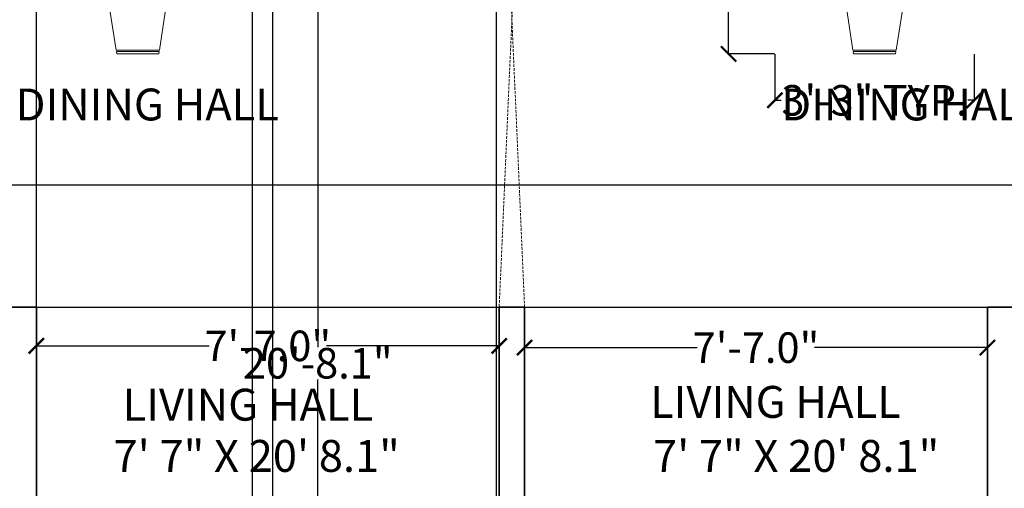
# Model space of a CAD drawing. Units: inches. Extents: x 844 to 2234, y 346 to 1084.
# Tile 42 of 93: x 1093 to 1287, y 731 to 823. Entities that reach past the tile are written whole.
import ezdxf

# ---------------------------------------------------------------- set-up
doc = ezdxf.new("R2010")
doc.units = ezdxf.units.IN
doc.header["$MEASUREMENT"] = 0
doc.linetypes.add('DASHED', pattern=[0.75, 0.5, -0.25])
for name, color, linetype, lineweight in [('A-ANNO-DIMS', 2, 'Continuous', 18), ('A-AREA-IDEN', 7, 'Continuous', 18), ('A-WALL', 7, 'Continuous', 35), ('A-WALL-OVHD', 7, 'DASHED', 18), ('furniture', 8, 'Continuous', 18)]:
    doc.layers.add(name, color=color, linetype=linetype, lineweight=lineweight)
doc.styles.add('ATTR', font='romans.shx', dxfattribs={"width": 0.8, "height": 0.7})
doc.styles.get("Standard").update_dxf_attribs({"font": 'arial.ttf'})
doc.dimstyles.get("Standard").update_dxf_attribs({"dimtxt": 6, "dimasz": 3, "dimexe": 0.18, "dimexo": 0.0625, "dimgap": 0.09, "dimtad": 0, "dimtih": 1, "dimtoh": 1, "dimdec": 1, "dimzin": 0, "dimdsep": 46, "dimlunit": 3, "dimtxsty": 'Standard', "dimblk": 'ARCHTICK', "dimcen": 0.09, "dimadec": 0, "dimazin": 0, "dimtfac": 1, "dimtdec": 1, "dimtofl": 0, "dimtmove": 0, "dimatfit": 3, "dimfxl": 1, "dimtolj": 1, "dimtzin": 0, "dimarcsym": 0})

# ---------------------------------------------------------------- blocks, each defined once
blk = doc.blocks.new('DIN42X84')
for p, q in [((-34.5377, 37.999999), (-34.6939, 37.000439)), ((-34.5377, 37.999999), (-18.5377, 37.999999)), ((-18.3814, 36.999659), (-18.5377, 37.999999)), ((-8.0001, 37.999999), (-8.1562, 37.000439)), ((-8.0001, 37.999999), (7.9999, 37.999999)), ((8.1562, 36.999659), (7.9999, 37.999999)), ((18.3813, 36.999659), (18.5376, 37.999999)), ((34.5376, 37.999999), (18.5376, 37.999999)), ((34.5376, 37.999999), (34.6938, 37.000439)), ((-34.772, 36.500609), (-37.0377, 21.999999)), ((-34.7681, 36.499999), (-18.2986, 36.499999)), ((-18.3793, 36.999999), (-34.6911, 36.999999)), ((-16.0377, 21.999999), (-18.3032, 36.499269)), ((-8.2343, 36.500609), (-10.5001, 21.999999)), ((-8.2305, 36.499999), (8.2391, 36.499999)), ((8.1584, 36.999999), (-8.1535, 36.999999)), ((10.4999, 21.999999), (8.2344, 36.499269)), ((16.0376, 21.999999), (18.3031, 36.499269)), ((34.768, 36.499999), (18.2985, 36.499999)), ((18.3792, 36.999999), (34.691, 36.999999)), ((34.7719, 36.500609), (37.0376, 21.999999)), ((-57.9997, 8.156299), (-59, 7.999989)), ((-59, -8.000011), (-59, 7.999989)), ((-58, 8.158429), (-58, -8.153391)), ((-57.5, -8.230411), (-57.5, 8.239139)), ((-43, 10.499989), (-57.4993, 8.234489)), ((43, 10.499989), (57.4992, 8.234489)), ((57.5, -8.230411), (57.5, 8.239139)), ((57.9996, 8.156299), (59, 7.999989)), ((58, 8.158429), (58, -8.153391)), ((59, -8.000011), (59, 7.999989)), ((-59, -8.000011), (-58.0005, -8.156181)), ((-57.5007, -8.234271), (-43, -10.500011)), ((57.5006, -8.234271), (43, -10.500011)), ((59, -8.000011), (58.0004, -8.156181)), ((-42, -21.000001), (42, -21.000001)), ((-34.772, -36.50061), (-37.0377, -22.000001)), ((-16.0377, -22.000001), (-18.3032, -36.499267)), ((-8.2343, -36.50061), (-10.5001, -22.000001)), ((10.4999, -22.000001), (8.2344, -36.499267)), ((16.0376, -22.000001), (18.3031, -36.499267)), ((34.7719, -36.50061), (37.0376, -22.000001)), ((-34.7681, -36.499999), (-18.2986, -36.499999)), ((-34.5377, -37.999999), (-34.6939, -37.000442)), ((-18.3793, -36.999999), (-34.6911, -36.999999)), ((-18.3814, -36.999664), (-18.5377, -37.999999)), ((-8.2305, -36.499999), (8.2391, -36.499999)), ((-8.0001, -37.999999), (-8.1562, -37.000442)), ((8.1584, -36.999999), (-8.1535, -36.999999)), ((8.1562, -36.999664), (7.9999, -37.999999)), ((34.768, -36.499999), (18.2985, -36.499999)), ((18.3792, -36.999999), (34.691, -36.999999)), ((18.3813, -36.999664), (18.5376, -37.999999)), ((34.5376, -37.999999), (34.6938, -37.000442)), ((-34.5377, -37.999999), (-18.5377, -37.999999)), ((-8.0001, -37.999999), (7.9999, -37.999999)), ((34.5376, -37.999999), (18.5376, -37.999999))]:
    blk.add_line(p, q)
for points in [[(-42, -21.000001), (-42, 20.999989), (42, 20.999989), (42, -21.000001)], [(-42, 16.999989), (-40.5974, 16.672209), (-39.2569, 16.395939), (-37.9668, 16.166109), (-36.7153, 15.977689), (-35.4906, 15.825599), (-34.281, 15.704799), (-33.0745, 15.610229), (-31.8595, 15.536839), (-30.6267, 15.480229), (-29.3778, 15.438619), (-28.117, 15.410889), (-26.8486, 15.395929), (-25.5767, 15.392599), (-24.3058, 15.399809), (-23.0399, 15.416409), (-21.7833, 15.441309), (-20.5384, 15.473619), (-19.2994, 15.513549), (-18.0587, 15.561549), (-16.8087, 15.618049), (-15.5417, 15.683499), (-14.25, 15.758369), (-12.9261, 15.843079), (-11.5622, 15.938089), (-10.1541, 16.043559), (-8.7108, 16.158419), (-7.2445, 16.281349), (-5.7675, 16.410999), (-4.2923, 16.546019), (-2.8311, 16.685069), (-1.3963, 16.826809), (0, 16.969889), (1.3474, 17.113339), (2.6447, 17.257689), (3.8928, 17.403829), (5.0924, 17.552659), (6.2444, 17.705069), (7.3498, 17.861959), (8.4092, 18.024219), (9.4237, 18.192759), (10.3952, 18.367629), (11.3311, 18.545639), (12.2397, 18.722759), (13.1297, 18.894949), (14.0095, 19.058179), (14.8876, 19.208429), (15.7725, 19.341659), (16.6727, 19.453839), (17.5977, 19.541909), (18.5617, 19.606689), (19.5795, 19.649979), (20.6664, 19.673569), (21.8374, 19.679239), (23.1076, 19.668789), (24.492, 19.644009), (26.0058, 19.606689), (27.6589, 19.554579), (29.4413, 19.469229), (31.3377, 19.328169), (33.3331, 19.108889), (35.4121, 18.788919), (37.5598, 18.345779), (39.7608, 17.756959), (42, 16.999989)], [(42, 12.999999), (39.3635, 13.704689), (36.9303, 14.232849), (34.6868, 14.608169), (32.6195, 14.854319), (30.7149, 14.994989), (28.9596, 15.053859), (27.34, 15.054629), (25.8427, 15.020959), (24.4543, 14.972439), (23.1628, 14.912279), (21.9562, 14.839589), (20.8227, 14.753449), (19.7504, 14.652989), (18.7273, 14.537299), (17.7416, 14.405489), (16.7814, 14.256669), (15.8348, 14.090369), (14.8899, 13.907959), (13.9348, 13.711209), (12.9575, 13.501929), (11.9464, 13.281899), (10.8893, 13.052909), (9.7745, 12.816759), (8.59, 12.575229), (7.3261, 12.330049), (5.9815, 12.082619), (4.557, 11.834299), (3.0536, 11.586429), (1.472, 11.340349), (-0.187, 11.097409), (-1.9223, 10.858939), (-3.7333, 10.626289), (-5.6141, 10.400739), (-7.539, 10.183249), (-9.4776, 9.974709), (-11.3991, 9.776019), (-13.2731, 9.588079), (-15.0689, 9.411789), (-16.756, 9.248039), (-18.3038, 9.097709), (-19.6928, 8.961719), (-20.9483, 8.840959), (-22.1065, 8.736319), (-23.2037, 8.648689), (-24.2763, 8.578979), (-25.3606, 8.528079), (-26.4928, 8.496879), (-27.7094, 8.486279), (-29.0411, 8.496689), (-30.4965, 8.526549), (-32.0787, 8.573829), (-33.7908, 8.636479), (-35.6359, 8.712459), (-37.6171, 8.799739), (-39.7374, 8.896259), (-42, 8.999999)], [(-42, 0.999999), (-39.2567, 1.059739), (-36.6668, 1.127399), (-34.2177, 1.203389), (-31.897, 1.288099), (-29.6923, 1.381949), (-27.5912, 1.485329), (-25.5812, 1.598659), (-23.65, 1.722319), (-21.7874, 1.856519), (-19.9935, 2.000569), (-18.2704, 2.153579), (-16.6207, 2.314649), (-15.0465, 2.482879), (-13.5503, 2.657379), (-12.1344, 2.837259), (-10.8011, 3.021619), (-9.5514, 3.209479), (-8.3812, 3.399579), (-7.2848, 3.590579), (-6.2569, 3.781129), (-5.2918, 3.969889), (-4.384, 4.155509), (-3.5281, 4.336659), (-2.7184, 4.511979), (-1.9505, 4.680359), (-1.2233, 4.841579), (-0.5369, 4.995629), (0.1087, 5.142519), (0.7135, 5.282239), (1.2776, 5.414799), (1.8009, 5.540189), (2.2834, 5.658409), (2.7259, 5.769699), (3.1323, 5.875159), (3.5073, 5.976139), (3.8555, 6.073989), (4.1816, 6.170049), (4.4904, 6.265659), (4.7863, 6.362169), (5.0742, 6.460919), (5.3584, 6.563099), (5.6417, 6.669299), (5.9267, 6.779989), (6.216, 6.895609), (6.512, 7.016589), (6.8174, 7.143399), (7.1347, 7.276479), (7.4664, 7.416279), (7.8159, 7.563169), (8.1896, 7.717219), (8.5948, 7.878439), (9.0386, 8.046819), (9.5282, 8.222369), (10.071, 8.405079), (10.674, 8.594959), (11.3446, 8.791999), (12.0866, 8.995459), (12.8902, 9.201609), (13.7421, 9.405969), (14.6294, 9.604059), (15.5387, 9.791399), (16.4569, 9.963509), (17.3709, 10.115919), (18.2674, 10.244149), (19.1361, 10.344989), (19.9772, 10.420299), (20.7936, 10.473209), (21.5884, 10.506879), (22.3645, 10.524419), (23.1248, 10.528969), (23.8725, 10.523669), (24.6103, 10.511649), (25.3403, 10.495379), (26.0601, 10.474629), (26.7663, 10.448509), (27.4556, 10.416119), (28.1244, 10.376559), (28.7695, 10.328939), (29.3873, 10.272359), (29.9746, 10.205939), (30.5293, 10.129059), (31.0552, 10.042329), (31.5572, 9.946639), (32.0406, 9.842899), (32.5104, 9.731989), (32.9716, 9.614799), (33.4295, 9.492249), (33.8891, 9.365219), (34.3546, 9.234229), (34.8266, 9.098309), (35.3051, 8.956129), (35.7897, 8.806329), (36.2802, 8.647569), (36.7765, 8.478519), (37.2783, 8.297819), (37.7854, 8.104139), (38.2976, 7.894309), (38.8146, 7.657969), (39.3361, 7.382899), (39.8617, 7.056919), (40.3912, 6.667829), (40.9243, 6.203449), (41.4607, 5.651569), (42, 4.999999)], [(42, 0.999999), (35.1214, 2.295539), (25.1178, 2.983399), (7.9376, 2.295539), (0.3261, 1.149099), (-6.6329, -0.226611), (-18.3763, -2.978061), (-22.0733, -3.895201), (-27.5101, -4.583071), (-32.9468, -4.583071), (-35.339, -4.583071), (-38.3836, -4.353771), (-40.3408, -3.665921), (-42, -3.000001)], [(42, -3.000001), (38.9344, -2.781351), (35.8829, -2.650251), (32.8567, -2.595491), (29.8672, -2.605821), (26.9257, -2.670031), (24.0436, -2.776881), (21.2323, -2.915141), (18.5031, -3.073591), (15.8668, -3.242611), (13.3327, -3.419021), (10.9095, -3.601241), (8.6059, -3.787731), (6.4305, -3.976901), (4.3921, -4.167191), (2.4994, -4.357031), (0.7611, -4.544851), (-0.8196, -4.729651), (-2.2614, -4.912671), (-3.5885, -5.095681), (-4.8252, -5.280481), (-5.9956, -5.468861), (-7.1239, -5.662621), (-8.2344, -5.863551), (-9.3513, -6.073431), (-10.4925, -6.293091), (-11.6511, -6.519461), (-12.814, -6.748531), (-13.968, -6.976251), (-15.0999, -7.198591), (-16.1965, -7.411531), (-17.2447, -7.611041), (-18.2313, -7.793081), (-19.1472, -7.954521), (-19.9994, -8.095811), (-20.7989, -8.218291), (-21.5568, -8.323311), (-22.2841, -8.412201), (-22.9919, -8.486311), (-23.6912, -8.546991), (-24.393, -8.595581), (-25.1087, -8.632751), (-25.8513, -8.656491), (-26.6337, -8.664101), (-27.4693, -8.652901), (-28.3711, -8.620211), (-29.3523, -8.563341), (-30.4262, -8.479601), (-31.6057, -8.366301), (-32.8956, -8.222561), (-34.2657, -8.054761), (-35.6772, -7.871051), (-37.0913, -7.679611), (-38.4695, -7.488621), (-39.7728, -7.306241), (-40.9626, -7.140641), (-42, -7.000001)], [(-42, -15.000001), (-38.4722, -15.350691), (-35.3039, -15.623741), (-32.4544, -15.828971), (-29.8831, -15.976191), (-27.5493, -16.075201), (-25.4123, -16.135831), (-23.4313, -16.167881), (-21.5659, -16.181151), (-19.7812, -16.183881), (-18.0665, -16.177871), (-16.4173, -16.163351), (-14.8288, -16.140551), (-13.2964, -16.109691), (-11.8154, -16.070991), (-10.3811, -16.024671), (-8.9888, -15.970971), (-7.6345, -15.909991), (-6.3163, -15.841401), (-5.0329, -15.764751), (-3.7831, -15.679591), (-2.5656, -15.585471), (-1.3791, -15.481951), (-0.2223, -15.368571), (0.9061, -15.244901), (2.0079, -15.110631), (3.0876, -14.966051), (4.1503, -14.811631), (5.2011, -14.647801), (6.2451, -14.475011), (7.2875, -14.293721), (8.3332, -14.104361), (9.3874, -13.907391), (10.4544, -13.703711), (11.5349, -13.495991), (12.6291, -13.287381), (13.7368, -13.081011), (14.8581, -12.880011), (15.9931, -12.687521), (17.1416, -12.506671), (18.3037, -12.340601), (19.4778, -12.191771), (20.6562, -12.059961), (21.8295, -11.944271), (22.9884, -11.843811), (24.1234, -11.757681), (25.2254, -11.684981), (26.2848, -11.624831), (27.2925, -11.576311), (28.2412, -11.538551), (29.1325, -11.510631), (29.9703, -11.491671), (30.7584, -11.480781), (31.5007, -11.477041), (32.2009, -11.479581), (32.8628, -11.487491), (33.4904, -11.499881), (34.0874, -11.515741), (34.6576, -11.533621), (35.2049, -11.551941), (35.733, -11.569151), (36.2459, -11.583661), (36.7473, -11.593931), (37.2411, -11.598371), (37.7311, -11.595421), (38.2211, -11.583281), (38.7152, -11.559251), (39.2177, -11.520361), (39.7326, -11.463671), (40.2641, -11.386241), (40.8164, -11.285111), (41.3937, -11.157351), (42, -11.000001)]]:
    blk.add_lwpolyline(points)
for centre, start, end in [((-36.0377, 21.999999), 180, 270), ((-17.0377, 21.999999), 270, 0), ((-9.5001, 21.999999), 180, 270), ((9.4999, 21.999999), 270, 0), ((17.0376, 21.999999), 180, 270), ((36.0376, 21.999999), 270, 0), ((-43, 9.499989), 0.00000068, 90), ((43, 9.499989), 90, 180), ((-43, -9.500011), 270, 0.00000068), ((43, -9.500011), 180, 270), ((-36.0377, -22.000001), 90, 180), ((-17.0377, -22.000001), 0, 90), ((-9.5001, -22.000001), 90, 180), ((9.4999, -22.000001), 0, 90), ((17.0376, -22.000001), 90, 180), ((36.0376, -22.000001), 0, 90)]:
    blk.add_arc(centre, 1, start, end)
at = {"style": 'ATTR', "width": 0.8, "flags": 9}
blk.add_attdef('ESTCODE', (0, 0), '', height=0.7, dxfattribs=at)
blk = doc.blocks.new('_ArchTick')
at = {"color": 0, "linetype": 'ByBlock', "const_width": 0.15}
blk.add_lwpolyline([(-0.5, -0.5), (0.5, 0.5)], dxfattribs=at)
blk = doc.blocks.new('*D49')
at = {"layer": 'A-ANNO-DIMS', "color": 0, "lineweight": -2, "transparency": 16777216}
for p, q in [((1192.62, 758.39), (1192.62, 758.51)), ((1192.62, 758.33), (1226.58, 758.33)), ((1283.62, 758.33), (1249.65, 758.33)), ((1283.62, 758.39), (1283.62, 758.51))]:
    blk.add_line(p, q, dxfattribs=at)
at = {"layer": 'Defpoints', "color": 0, "transparency": 16777216}
for p in [(1192.62, 758.33), (1192.62, 758.33), (1283.62, 758.33)]:
    blk.add_point(p, dxfattribs=at)
at = {"layer": 'A-ANNO-DIMS', "color": 0, "lineweight": -2, "transparency": 16777216, "xscale": 3, "yscale": 3, "zscale": 3, "rotation": 180}
blk.add_blockref('_ArchTick', (1192.62, 758.33), dxfattribs=at)
at = {"layer": 'A-ANNO-DIMS', "color": 0, "lineweight": -2, "transparency": 16777216, "xscale": 3, "yscale": 3, "zscale": 3}
blk.add_blockref('_ArchTick', (1283.62, 758.33), dxfattribs=at)
at = {"layer": 'A-ANNO-DIMS', "color": 0, "transparency": 16777216, "insert": (1238.12, 758.33), "char_height": 6, "attachment_point": 5}
blk.add_mtext('\\A1;7\'-7.0"', dxfattribs=at)
blk = doc.blocks.new('*D53')
at = {"layer": 'A-ANNO-DIMS', "color": 0, "lineweight": -2, "transparency": 16777216}
for p, q in [((1096.62, 758.67), (1130.58, 758.67)), ((1096.62, 758.6), (1096.62, 758.49)), ((1187.62, 758.67), (1153.65, 758.67)), ((1187.62, 758.73), (1187.62, 758.85))]:
    blk.add_line(p, q, dxfattribs=at)
at = {"layer": 'Defpoints', "color": 0, "transparency": 16777216}
for p in [(1096.62, 758.67), (1187.62, 758.67), (1187.62, 758.67)]:
    blk.add_point(p, dxfattribs=at)
at = {"layer": 'A-ANNO-DIMS', "color": 0, "lineweight": -2, "transparency": 16777216, "xscale": 3, "yscale": 3, "zscale": 3, "rotation": 180}
blk.add_blockref('_ArchTick', (1096.62, 758.67), dxfattribs=at)
at = {"layer": 'A-ANNO-DIMS', "color": 0, "lineweight": -2, "transparency": 16777216, "xscale": 3, "yscale": 3, "zscale": 3}
blk.add_blockref('_ArchTick', (1187.62, 758.67), dxfattribs=at)
at = {"layer": 'A-ANNO-DIMS', "color": 0, "transparency": 16777216, "insert": (1142.12, 758.67), "char_height": 6, "attachment_point": 5}
blk.add_mtext('\\A1;7\'-7.0"', dxfattribs=at)
blk = doc.blocks.new('*D54')
at = {"layer": 'A-ANNO-DIMS', "color": 0, "lineweight": -2, "transparency": 16777216}
for p, q in [((1139.68, 879.31), (1152.12, 879.31)), ((1151.94, 879.31), (1151.94, 758.4)), ((1151.94, 631.18), (1151.94, 752.09)), ((1139.68, 631.18), (1152.12, 631.18))]:
    blk.add_line(p, q, dxfattribs=at)
at = {"layer": 'Defpoints', "color": 0, "transparency": 16777216}
for p in [(1139.62, 879.31), (1139.62, 631.18), (1151.94, 631.18)]:
    blk.add_point(p, dxfattribs=at)
at = {"layer": 'A-ANNO-DIMS', "color": 0, "lineweight": -2, "transparency": 16777216, "xscale": 3, "yscale": 3, "zscale": 3}
for p, rotation in [((1151.94, 879.31), 90), ((1151.94, 631.18), 270)]:
    blk.add_blockref('_ArchTick', p, dxfattribs=dict(at, rotation=rotation))
at = {"layer": 'A-ANNO-DIMS', "color": 0, "transparency": 16777216, "insert": (1151.94, 755.25), "char_height": 6, "attachment_point": 5}
blk.add_mtext('\\A1;20\'-8.1"', dxfattribs=at)
blk = doc.blocks.new('*D119')
at = {"layer": 'A-ANNO-DIMS', "color": 0, "lineweight": -2, "transparency": 16777216}
for p, q in [((1241.78, 876.89), (1232.54, 876.89)), ((1232.72, 876.89), (1232.72, 849.68)), ((1232.72, 816.08), (1232.72, 843.29)), ((1241.78, 816.08), (1232.54, 816.08))]:
    blk.add_line(p, q, dxfattribs=at)
at = {"layer": 'Defpoints', "color": 0, "transparency": 16777216}
for p in [(1232.72, 876.89), (1241.84, 876.89), (1241.84, 816.08)]:
    blk.add_point(p, dxfattribs=at)
at = {"layer": 'A-ANNO-DIMS', "color": 0, "lineweight": -2, "transparency": 16777216, "xscale": 3, "yscale": 3, "zscale": 3}
for p, rotation in [((1232.72, 876.89), 90), ((1232.72, 816.08), 270)]:
    blk.add_blockref('_ArchTick', p, dxfattribs=dict(at, rotation=rotation))
at = {"layer": 'A-ANNO-DIMS', "color": 0, "transparency": 16777216, "insert": (1232.72, 846.48), "char_height": 6, "attachment_point": 5}
blk.add_mtext('\\A1;DINING SET 5\'-1" TYP.', dxfattribs=at)
blk = doc.blocks.new('*D120')
at = {"layer": 'A-ANNO-DIMS', "color": 0, "lineweight": -2, "transparency": 16777216}
for p, q in [((1241.84, 816.01), (1241.84, 806.78)), ((1281.01, 816.01), (1281.01, 806.78)), ((1241.84, 806.96), (1243.05, 806.96)), ((1281.01, 806.96), (1279.8, 806.96))]:
    blk.add_line(p, q, dxfattribs=at)
at = {"layer": 'Defpoints', "color": 0, "transparency": 16777216}
for p in [(1241.84, 816.08), (1281.01, 816.08), (1241.84, 806.96)]:
    blk.add_point(p, dxfattribs=at)
at = {"layer": 'A-ANNO-DIMS', "color": 0, "lineweight": -2, "transparency": 16777216, "xscale": 3, "yscale": 3, "zscale": 3, "rotation": 180}
blk.add_blockref('_ArchTick', (1241.84, 806.96), dxfattribs=at)
at = {"layer": 'A-ANNO-DIMS', "color": 0, "lineweight": -2, "transparency": 16777216, "xscale": 3, "yscale": 3, "zscale": 3}
blk.add_blockref('_ArchTick', (1281.01, 806.96), dxfattribs=at)
at = {"layer": 'A-ANNO-DIMS', "color": 0, "transparency": 16777216, "insert": (1261.43, 806.96), "char_height": 6, "attachment_point": 5}
blk.add_mtext('\\A1;3\'-3" TYP.', dxfattribs=at)
blk = doc.blocks.new('*D143')
at = {"layer": 'A-ANNO-DIMS', "color": 0, "lineweight": -2, "transparency": 16777216}
for p, q in [((1139.12, 430.37), (1139.12, 1074.74)), ((1139.12, 1074.56), (1154.93, 1074.56)), ((1187.12, 1074.56), (1171.3, 1074.56)), ((1187.12, 430.37), (1187.12, 1074.74))]:
    blk.add_line(p, q, dxfattribs=at)
at = {"layer": 'Defpoints', "color": 0, "transparency": 16777216}
for p in [(1187.12, 1074.56), (1139.12, 430.31), (1187.12, 430.31)]:
    blk.add_point(p, dxfattribs=at)
at = {"layer": 'A-ANNO-DIMS', "color": 0, "lineweight": -2, "transparency": 16777216, "xscale": 3, "yscale": 3, "zscale": 3, "rotation": 180}
blk.add_blockref('_ArchTick', (1139.12, 1074.56), dxfattribs=at)
at = {"layer": 'A-ANNO-DIMS', "color": 0, "lineweight": -2, "transparency": 16777216, "xscale": 3, "yscale": 3, "zscale": 3}
blk.add_blockref('_ArchTick', (1187.12, 1074.56), dxfattribs=at)
at = {"layer": 'A-ANNO-DIMS', "color": 0, "transparency": 16777216, "insert": (1163.12, 1074.56), "char_height": 6, "attachment_point": 5}
blk.add_mtext('\\A1;4\'-0"', dxfattribs=at)
blk = doc.blocks.new('*D144')
at = {"layer": 'A-ANNO-DIMS', "color": 0, "lineweight": -2, "transparency": 16777216}
for p, q in [((1096.62, 439.37), (1096.62, 1074.74)), ((1096.62, 1074.56), (1102.48, 1074.56)), ((1143.12, 1074.56), (1137.25, 1074.56)), ((1143.12, 492.37), (1143.12, 1074.74))]:
    blk.add_line(p, q, dxfattribs=at)
at = {"layer": 'Defpoints', "color": 0, "transparency": 16777216}
for p in [(1143.12, 1074.56), (1143.12, 492.31), (1096.62, 439.31)]:
    blk.add_point(p, dxfattribs=at)
at = {"layer": 'A-ANNO-DIMS', "color": 0, "lineweight": -2, "transparency": 16777216, "xscale": 3, "yscale": 3, "zscale": 3, "rotation": 180}
blk.add_blockref('_ArchTick', (1096.62, 1074.56), dxfattribs=at)
at = {"layer": 'A-ANNO-DIMS', "color": 0, "lineweight": -2, "transparency": 16777216, "xscale": 3, "yscale": 3, "zscale": 3}
blk.add_blockref('_ArchTick', (1143.12, 1074.56), dxfattribs=at)
at = {"layer": 'A-ANNO-DIMS', "color": 0, "transparency": 16777216, "insert": (1119.87, 1074.56), "char_height": 6, "attachment_point": 5}
blk.add_mtext('\\A1;3\'-10 1/2"', dxfattribs=at)
blk = doc.blocks.new('*D149')
at = {"layer": 'A-ANNO-DIMS', "color": 0, "lineweight": -2, "transparency": 16777216}
for p, q in [((1043.68, 790.31), (1479.05, 790.31)), ((1478.87, 790.31), (1478.87, 781.46)), ((1478.87, 766.31), (1478.87, 775.16)), ((1043.68, 766.31), (1479.05, 766.31))]:
    blk.add_line(p, q, dxfattribs=at)
at = {"layer": 'Defpoints', "color": 0, "transparency": 16777216}
for p in [(1043.62, 790.31), (1478.87, 790.31), (1043.62, 766.31)]:
    blk.add_point(p, dxfattribs=at)
at = {"layer": 'A-ANNO-DIMS', "color": 0, "lineweight": -2, "transparency": 16777216, "xscale": 3, "yscale": 3, "zscale": 3}
for p, rotation in [((1478.87, 790.31), 90), ((1478.87, 766.31), 270)]:
    blk.add_blockref('_ArchTick', p, dxfattribs=dict(at, rotation=rotation))
at = {"layer": 'A-ANNO-DIMS', "color": 0, "transparency": 16777216, "insert": (1478.87, 778.31), "char_height": 6, "attachment_point": 5}
blk.add_mtext('\\A1;2\'-0"', dxfattribs=at)

msp = doc.modelspace()

# ---------------------------------------------------------------- linework, layer by layer
at = {"layer": 'A-WALL'}
for p, q in [((1091.62, 766.31), (1096.62, 766.31)), ((1096.62, 761.31), (1096.62, 766.31)), ((1187.62, 766.31), (1192.62, 766.31)), ((1187.62, 766.31), (1187.62, 629.31)), ((1192.62, 766.31), (1192.62, 629.31)), ((1283.62, 761.31), (1283.62, 766.31)), ((1288.62, 766.31), (1283.62, 766.31)), ((1096.62, 761.31), (1096.62, 624.31)), ((1283.62, 761.31), (1283.62, 624.31))]:
    msp.add_line(p, q, dxfattribs=at)
at = {"layer": 'A-WALL-OVHD'}
for p, q in [((1192.62, 766.31), (1187.62, 879.31)), ((1192.62, 879.31), (1187.62, 766.31))]:
    msp.add_line(p, q, dxfattribs=at)

# ---------------------------------------------------------------- block references
at = {"layer": 'furniture', "xscale": 0.5153672157522483, "yscale": 0.5153672157522483, "zscale": 0.5153672157522483, "rotation": 90}
for p in [(1116.56, 846.48), (1261.43, 846.48)]:
    msp.add_blockref('DIN42X84', p, dxfattribs=at)

# ---------------------------------------------------------------- texts
at = {"layer": 'A-AREA-IDEN'}
for s, p in [('DINING HALL', (1092.53, 803)), ('DINING HALL', (1243.09, 803)), ('LIVING HALL', (1113.58, 743.97)), ('  LIVING HALL', (1213.47, 744.52)), (' 7\' 7" X 20\' 8.1"', (1109.88, 733.9)), (' 7\' 7" X 20\' 8.1"', (1215.96, 733.9))]:
    msp.add_text(s, height=6.2688, dxfattribs=at).set_placement(p)

# ---------------------------------------------------------------- dimensions: what is measured, and where the dimension line sits
at = {"layer": 'A-ANNO-DIMS'}
for base, p1, p2, override, picture, middle in [((1143.12, 1074.56), (1096.62, 439.31), (1143.12, 492.31), {"dimdec": 1, "dimlfac": 1, "dimrnd": 0, "dimzin": 1, "dimdsep": 46, "dimlunit": 4, "dimfrac": 2}, '*D144', (1119.87, 1074.56)), ((1187.12, 1074.56), (1139.12, 430.31), (1187.12, 430.31), {"dimdec": 1, "dimlfac": 1, "dimrnd": 0, "dimzin": 1, "dimdsep": 46, "dimlunit": 4, "dimfrac": 2}, '*D143', (1163.12, 1074.56)), ((1187.62, 758.67), (1096.62, 758.67), (1187.62, 758.67), {"dimclrd": 0, "dimclre": 0, "dimclrt": 0}, '*D53', (1142.12, 758.67)), ((1192.62, 758.33), (1283.62, 758.33), (1192.62, 758.33), {"dimclrd": 0, "dimclre": 0, "dimclrt": 0}, '*D49', (1238.12, 758.33))]:
    dim = msp.add_linear_dim(base=base, p1=p1, p2=p2, dimstyle='Standard', override=override, dxfattribs=at)
    dim.commit()
    dim.dimension.update_dxf_attribs({"geometry": picture, "text_midpoint": middle})
for base, p1, p2, override, picture, middle in [((1151.94, 631.18), (1139.62, 879.31), (1139.62, 631.18), {"dimclrd": 0, "dimclre": 0, "dimclrt": 0}, '*D54', (1151.94, 755.25)), ((1478.87, 790.31), (1043.62, 766.31), (1043.62, 790.31), {"dimdec": 1, "dimlfac": 1, "dimrnd": 0, "dimzin": 1, "dimdsep": 46, "dimlunit": 4, "dimfrac": 2}, '*D149', (1478.87, 778.31))]:
    dim = msp.add_linear_dim(base=base, p1=p1, p2=p2, angle=90, dimstyle='Standard', override=override, dxfattribs=at)
    dim.commit()
    dim.dimension.update_dxf_attribs({"geometry": picture, "text_midpoint": middle})
for base, p1, p2, angle, text, picture, middle in [((1232.72, 876.89), (1241.84, 816.08), (1241.84, 876.89), 90, 'DINING SET <> TYP.', '*D119', (1232.72, 846.48)), ((1241.84, 806.96), (1281.01, 816.08), (1241.84, 816.08), 180, '<> TYP.', '*D120', (1261.43, 806.96))]:
    dim = msp.add_linear_dim(base=base, p1=p1, p2=p2, angle=angle, text=text, dimstyle='Standard', override={"dimdec": 1, "dimlfac": 1, "dimrnd": 0, "dimzin": 1, "dimdsep": 46, "dimlunit": 4, "dimfrac": 2}, dxfattribs=at)
    dim.commit()
    dim.dimension.update_dxf_attribs({"geometry": picture, "text_midpoint": middle})

doc.saveas('drawing.dxf')
